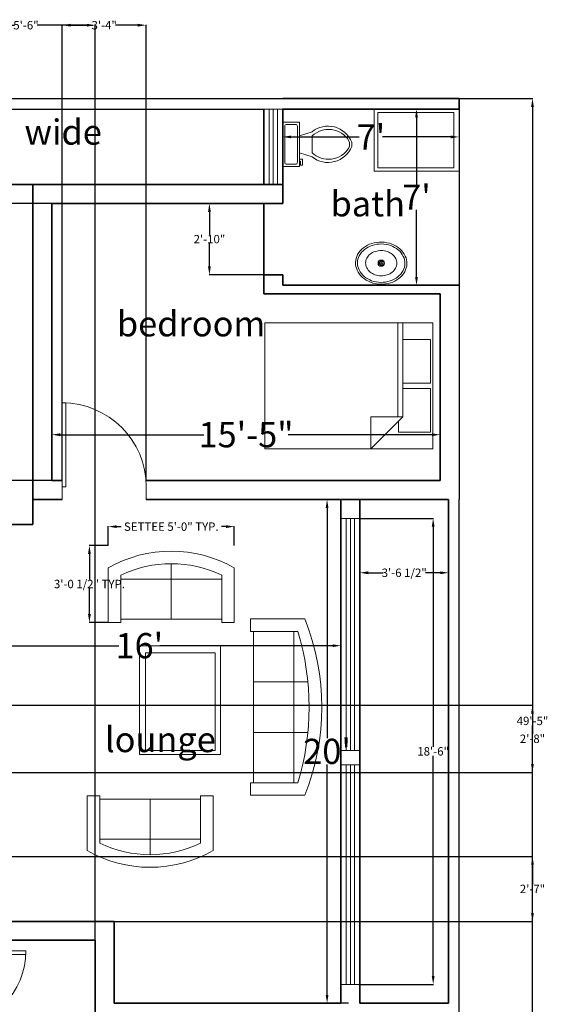
# Model space of a CAD drawing. Units: inches. Extents: x -346 to 220, y 97 to 877.
# Tile 4 of 4: x -32 to 220, y 404 to 873. Entities that reach past the tile are written whole.
import ezdxf

# ---------------------------------------------------------------- set-up
doc = ezdxf.new("R2010")
doc.units = ezdxf.units.IN
doc.header["$MEASUREMENT"] = 0
doc.layers.get('0').update_dxf_attribs({"color": 3})
for name, color, linetype, lineweight in [('A-AREA-IDEN', 130, 'Continuous', 25), ('A-FLOR-FIXT', 9, 'Continuous', 18), ('A-FURN', 8, 'Continuous', 18), ('A-WALL', 7, 'Continuous', 35), ('C-PROP', 94, 'Continuous', 25), ('dim', 170, 'Continuous', 13), ('door', 20, 'Continuous', 18), ('window', 230, 'Continuous', 18)]:
    doc.layers.add(name, color=color, linetype=linetype, lineweight=lineweight)
doc.styles.get("Standard").update_dxf_attribs({"font": 'arial.ttf'})
doc.dimstyles.get("Standard").update_dxf_attribs({"dimtxt": 4, "dimasz": 4, "dimexe": 0.18, "dimexo": 0.0625, "dimgap": 0.09, "dimtad": 0, "dimtih": 1, "dimtoh": 1, "dimdec": 0, "dimzin": 0, "dimdsep": 46, "dimlunit": 3, "dimtxsty": 'Standard', "dimcen": 0.09, "dimadec": 0, "dimazin": 0, "dimtfac": 1, "dimtdec": 0, "dimtofl": 0, "dimtmove": 0, "dimatfit": 3, "dimfxl": 1, "dimtolj": 1, "dimtzin": 0, "dimarcsym": 0})

# ---------------------------------------------------------------- blocks, each defined once
blk = doc.blocks.new('*D2')
at = {"layer": 'Defpoints', "color": 0, "transparency": 16777216}
for p in [(-16.93, 675.59), (-16.93, 653.75), (168.07, 653.75)]:
    blk.add_point(p, dxfattribs=at)
at = {"layer": 'dim', "color": 0, "lineweight": -2, "transparency": 16777216}
for p, q in [((-16.93, 653.81), (-16.93, 675.77)), ((-12.93, 675.59), (55.44, 675.59)), ((164.07, 675.59), (95.71, 675.59)), ((168.07, 653.81), (168.07, 675.77))]:
    blk.add_line(p, q, dxfattribs=at)
at = {"layer": 'dim', "color": 0, "transparency": 16777216}
for points in [[(-12.93, 676.25), (-12.93, 674.92), (-16.93, 675.59)], [(164.07, 676.25), (164.07, 674.92), (168.07, 675.59)]]:
    blk.add_solid(points, dxfattribs=at)
at = {"layer": 'dim', "color": 0, "transparency": 16777216, "insert": (75.57, 675.59), "char_height": 4, "attachment_point": 5}
blk.add_mtext('\\A1;{\\H3x;15\'-5"}', dxfattribs=at)
blk = doc.blocks.new('*D3')
at = {"layer": 'Defpoints', "color": 0, "transparency": 16777216}
for p in [(93.07, 826.04), (177.07, 826.04), (177.07, 817.44)]:
    blk.add_point(p, dxfattribs=at)
at = {"layer": 'dim', "color": 0, "lineweight": -2, "transparency": 16777216}
for p, q in [((93.07, 825.98), (93.07, 817.26)), ((177.07, 825.98), (177.07, 817.26)), ((97.07, 817.44), (129.51, 817.44)), ((173.07, 817.44), (140.63, 817.44))]:
    blk.add_line(p, q, dxfattribs=at)
at = {"layer": 'dim', "color": 0, "transparency": 16777216}
for points in [[(97.07, 818.11), (97.07, 816.78), (93.07, 817.44)], [(173.07, 818.11), (173.07, 816.78), (177.07, 817.44)]]:
    blk.add_solid(points, dxfattribs=at)
at = {"layer": 'dim', "color": 0, "transparency": 16777216, "insert": (135.07, 817.44), "char_height": 4, "attachment_point": 5}
blk.add_mtext("\\A1;{\\H3x;7'}", dxfattribs=at)
blk = doc.blocks.new('*D4')
at = {"layer": 'Defpoints', "color": 0, "transparency": 16777216}
for p in [(177.07, 830.75), (156.76, 746.75), (177.07, 746.75)]:
    blk.add_point(p, dxfattribs=at)
at = {"layer": 'dim', "color": 0, "lineweight": -2, "transparency": 16777216}
for p, q in [((177.01, 830.75), (156.58, 830.75)), ((156.76, 826.75), (156.76, 794.84)), ((156.76, 750.75), (156.76, 782.66)), ((177.01, 746.75), (156.58, 746.75))]:
    blk.add_line(p, q, dxfattribs=at)
at = {"layer": 'dim', "color": 0, "transparency": 16777216}
for points in [[(156.09, 826.75), (157.42, 826.75), (156.76, 830.75)], [(156.09, 750.75), (157.42, 750.75), (156.76, 746.75)]]:
    blk.add_solid(points, dxfattribs=at)
at = {"layer": 'dim', "color": 0, "transparency": 16777216, "insert": (156.76, 788.75), "char_height": 4, "attachment_point": 5}
blk.add_mtext("\\A1;{\\H3x;7'}", dxfattribs=at)
blk = doc.blocks.new('*D5')
at = {"layer": 'Defpoints', "color": 0, "transparency": 16777216}
for p in [(124.4, 644.75), (114.18, 404.75), (124.4, 404.75)]:
    blk.add_point(p, dxfattribs=at)
at = {"layer": 'dim', "color": 0, "lineweight": -2, "transparency": 16777216}
for p, q in [((124.33, 644.75), (114, 644.75)), ((114.18, 640.75), (114.18, 530.96)), ((114.18, 408.75), (114.18, 518.53)), ((124.33, 404.75), (114, 404.75))]:
    blk.add_line(p, q, dxfattribs=at)
at = {"layer": 'dim', "color": 0, "transparency": 16777216}
for points in [[(113.52, 640.75), (114.85, 640.75), (114.18, 644.75)], [(113.52, 408.75), (114.85, 408.75), (114.18, 404.75)]]:
    blk.add_solid(points, dxfattribs=at)
at = {"layer": 'dim', "color": 0, "transparency": 16777216, "insert": (114.18, 524.75), "char_height": 4, "attachment_point": 5}
blk.add_mtext("\\A1;{\\H3x;20'}", dxfattribs=at)
blk = doc.blocks.new('*D6')
at = {"layer": 'Defpoints', "color": 0, "transparency": 16777216}
for p in [(120.77, 575.08), (-71.23, 560.75), (120.77, 560.75)]:
    blk.add_point(p, dxfattribs=at)
at = {"layer": 'dim', "color": 0, "lineweight": -2, "transparency": 16777216}
for p, q in [((-71.23, 560.81), (-71.23, 575.26)), ((-67.23, 575.08), (15.07, 575.08)), ((116.77, 575.08), (34.48, 575.08)), ((120.77, 560.81), (120.77, 575.26))]:
    blk.add_line(p, q, dxfattribs=at)
at = {"layer": 'dim', "color": 0, "transparency": 16777216}
for points in [[(-67.23, 575.75), (-67.23, 574.41), (-71.23, 575.08)], [(116.77, 575.75), (116.77, 574.41), (120.77, 575.08)]]:
    blk.add_solid(points, dxfattribs=at)
at = {"layer": 'dim', "color": 0, "transparency": 16777216, "insert": (24.77, 575.08), "char_height": 4, "attachment_point": 5}
blk.add_mtext("\\A1;{\\H3x;16'}", dxfattribs=at)
blk = doc.blocks.new('*U13')
for p, q in [((0, 0), (0, -6)), ((36, 0), (36, -6))]:
    blk.add_line(p, q)
blk.add_lwpolyline([(0, 0), (0, 36), (1.75, 36), (1.75, 0)], close=True)
blk.add_arc((0, 0), 36, 0, 90)
blk = doc.blocks.new('*U18')
for p, q in [((0, 0), (0, -6)), ((-40, 0), (-40, -6))]:
    blk.add_line(p, q)
blk.add_lwpolyline([(0, 0), (0, 40), (-1.75, 40), (-1.75, 0)], close=True)
blk.add_arc((0, 0), 40, 90, 180)
blk = doc.blocks.new('Bed - Queen')
for p, q in [((0, -80.00003), (0, 0)), ((0, 0), (59.99999, 0)), ((59.99999, 0), (59.99999, -80.00003)), ((7.99999, -1.2), (28.79998, -1.2)), ((7.99999, -14.4), (7.99999, -1.2)), ((28.79998, -1.2), (28.79998, -14.4)), ((31.19999, -1.2), (51.99999, -1.2)), ((31.19999, -14.4), (31.19999, -1.2)), ((51.99999, -1.2), (51.99999, -16.4)), ((0, -14.4), (44.8, -14.4)), ((44.8, -16.8), (0, -16.8)), ((59.99999, -29.6), (44.8, -14.4)), ((44.8, -14.4), (44.8, -29.6)), ((51.99999, -16.4), (46.79936, -16.4)), ((44.8, -29.6), (59.99999, -29.6)), ((59.99999, -80.00003), (0, -80.00003))]:
    blk.add_line(p, q)
blk = doc.blocks.new('Toilet - top')
for p, q in [((9.5, -6), (9.5, -2)), ((-10, -8.5), (-8, -8.5)), ((-10, -9.5), (-10, -8.5)), ((-8, -8.5), (-8, -8)), ((-7, -8), (-7, -9.5)), ((-4, -8), (-6, -14)), ((4, -8), (6, -14)), ((-7, -9.5), (-10, -9.5)), ((4, -14), (-4, -14))]:
    blk.add_line(p, q)
blk.add_lwpolyline([(10.5, -8), (10.5, 0), (-10.5, 0), (-10.5, -8)], close=True)
for points in [[(-9.5, -2), (-9.5, -6)], [(8.5, -1), (-8.5, -1)], [(-8.5, -7), (8.5, -7)]]:
    blk.add_lwpolyline(points)
for centre, radius, start, end in [((-8.62, -1.88), 0.884, 81.8699, 188.1301), ((8.62, -1.88), 0.884, 351.8699, 98.1301), ((-8.62, -6.12), 0.884, 171.8699, 278.1301), ((8.62, -6.12), 0.884, 261.8699, 8.1301), ((3.52, -21.58), 12.17, 141.4691, 247.9714), ((4.2, -21.82), 11.33, 136.3677, 238.9468), ((-3.52, -21.58), 12.17, 292.0284, 38.5307), ((-4.2, -21.82), 11.33, 301.053, 43.6321), ((0, -27.88), 4, 245.7318, 294.2682), ((0, -29), 4, 254.8605, 285.1395)]:
    blk.add_arc(centre, radius, start, end)
blk = doc.blocks.new('Sofa - Roundback 7 ft.')
for p, q in [((-12.00002, -32.4421), (-12.00003, -6.5971)), ((11.99997, -32.4421), (11.99998, -6.5971)), ((-36.000027, -34), (-36.000027, -11.4696)), ((-35.999844, -13.3819), (35.9998, -13.3819)), ((35.99998, -34), (35.99998, -11.4696)), ((-36.000027, -32.4421), (35.99998, -32.4421))]:
    blk.add_line(p, q)
for points in [[(-36.000027, -34), (-42.000027, -34), (-42.000027, -8)], [(41.99998, -8), (41.99998, -34), (35.99998, -34)]]:
    blk.add_lwpolyline(points)
for centre, radius, start, end in [((0, -114.25), 114.25, 68.43141, 111.5686), ((-0.00001, -127.1968), 121.1968, 72.72033, 107.2797)]:
    blk.add_arc(centre, radius, start, end)
blk = doc.blocks.new('Sofa - Roundback Loveseat 5 ft.')
for p, q in [((0, -32.44198), (0, -5.99998)), ((-24, -33.99998), (-24, -11.46958)), ((-23.9998, -13.38178), (23.99986, -13.38178)), ((24.00004, -33.99998), (24.00004, -11.46958)), ((-24, -32.44198), (24.00004, -32.44198))]:
    blk.add_line(p, q)
for points in [[(-24, -33.99998), (-30, -33.99998), (-30, -7.99998)], [(30.00004, -7.99998), (30.00004, -33.99998), (24.00004, -33.99998)]]:
    blk.add_lwpolyline(points)
for centre, radius, start, end in [((0, -60.24998), 60.24998, 60.13715, 119.8628), ((0, -61.38438), 55.38444, 64.32083, 115.6792)]:
    blk.add_arc(centre, radius, start, end)
blk = doc.blocks.new('Sink - Oval top')
for p, q in [((-1, 0), (1, 0)), ((0, 1), (0, -1))]:
    blk.add_line(p, q)
for points in [[(-12.23, 0.39, 0.117634), (-11.46, -3.36, 0.104469), (-8.88, -6.8, 0.090016), (-5.08, -9.07, 0.08192), (-0.32, -10.02, 0.08192), (4.49, -9.38, 0.090016), (8.42, -7.36, 0.104469), (11.22, -4.09, 0.117634), (12.23, -0.39, 0.117634), (11.46, 3.36, 0.104469), (8.88, 6.8, 0.090016), (5.08, 9.07, 0.08192), (0.32, 10.02, 0.08192), (-4.49, 9.38, 0.090016), (-8.42, 7.36, 0.104469), (-11.22, 4.09, 0.117634)], [(-11.29, 0.16, 0.118622), (-10.52, -3.25, 0.104678), (-8.07, -6.36, 0.089562), (-4.54, -8.37, 0.081185), (-0.13, -9.15, 0.081185), (4.3, -8.49, 0.089562), (7.89, -6.58, 0.104678), (10.42, -3.55, 0.118622), (11.29, -0.16, 0.118622), (10.52, 3.25, 0.104678), (8.07, 6.36, 0.089562), (4.54, 8.37, 0.081185), (0.13, 9.15, 0.081185), (-4.3, 8.49, 0.089562), (-7.89, 6.58, 0.104678), (-10.42, 3.55, 0.118622)], [(-7.42, 0.08, 0.118283), (-6.91, -2.17, 0.104607), (-5.29, -4.21, 0.089718), (-2.97, -5.53, 0.081436), (-0.07, -6.04, 0.081436), (2.84, -5.59, 0.089718), (5.2, -4.33, 0.104607), (6.86, -2.32, 0.118283), (7.42, -0.08, 0.118283), (6.91, 2.17, 0.104607), (5.29, 4.21, 0.089718), (2.97, 5.53, 0.081436), (0.07, 6.04, 0.081436), (-2.84, 5.59, 0.089718), (-5.2, 4.33, 0.104607), (-6.86, 2.32, 0.118283)]]:
    blk.add_lwpolyline(points, format="xyb", close=True)
for radius in [1.5, 1]:
    blk.add_circle((0, 0), radius)
blk = doc.blocks.new('WIN-36x9-PLAN')
for p, q in [((2.5, 36), (2.5, 0)), ((4.5, 36), (4.5, 0)), ((6.5, 36), (6.5, 0))]:
    blk.add_line(p, q)
blk.add_lwpolyline([(0, 36), (9, 36), (9, 0), (0, 0)], close=True)
blk = doc.blocks.new('TABLE-COFFEE-RECT')
for points in [[(0, 51.83), (38.64, 51.83), (38.64, 0), (0, 0)], [(2.97, 48.5), (36.03, 48.5), (36.03, 1.93), (2.97, 1.93)]]:
    blk.add_lwpolyline(points, close=True)
blk = doc.blocks.new('*D38')
at = {"layer": 'Defpoints', "color": 0, "transparency": 16777216}
for p in [(69.99, 631.8), (9.99, 622.8), (69.99, 622.8)]:
    blk.add_point(p, dxfattribs=at)
at = {"layer": 'dim', "color": 0, "lineweight": -2, "transparency": 16777216}
for p, q in [((9.99, 622.87), (9.99, 631.98)), ((13.99, 631.8), (16.07, 631.8)), ((65.99, 631.8), (63.9, 631.8)), ((69.99, 622.87), (69.99, 631.98))]:
    blk.add_line(p, q, dxfattribs=at)
at = {"layer": 'dim', "color": 0, "transparency": 16777216}
for points in [[(13.99, 632.47), (13.99, 631.14), (9.99, 631.8)], [(65.99, 632.47), (65.99, 631.14), (69.99, 631.8)]]:
    blk.add_solid(points, dxfattribs=at)
at = {"layer": 'dim', "color": 0, "transparency": 16777216, "insert": (39.99, 631.8), "char_height": 4, "attachment_point": 5}
blk.add_mtext('\\A1;SETTEE 5\'-0" TYP.', dxfattribs=at)
blk = doc.blocks.new('*D39')
at = {"layer": 'Defpoints', "color": 0, "transparency": 16777216}
for p in [(0.99, 622.8), (9.99, 622.8), (9.99, 586.14)]:
    blk.add_point(p, dxfattribs=at)
at = {"layer": 'dim', "color": 0, "lineweight": -2, "transparency": 16777216}
for p, q in [((9.92, 622.8), (0.81, 622.8)), ((0.99, 618.8), (0.99, 606.63)), ((0.99, 590.14), (0.99, 602.31)), ((9.92, 586.14), (0.81, 586.14))]:
    blk.add_line(p, q, dxfattribs=at)
at = {"layer": 'dim', "color": 0, "transparency": 16777216}
for points in [[(0.32, 618.8), (1.65, 618.8), (0.99, 622.8)], [(0.32, 590.14), (1.65, 590.14), (0.99, 586.14)]]:
    blk.add_solid(points, dxfattribs=at)
at = {"layer": 'dim', "color": 0, "transparency": 16777216, "insert": (0.99, 604.47), "char_height": 4, "attachment_point": 5}
blk.add_mtext('\\A1;3\'-0 1/2" TYP.', dxfattribs=at)
blk = doc.blocks.new('*D51')
at = {"layer": 'Defpoints', "color": 0, "transparency": 16777216}
for p in [(177.07, 835.75), (212, 835.75), (177.07, 242.75)]:
    blk.add_point(p, dxfattribs=at)
at = {"layer": 'dim', "color": 0, "lineweight": -2, "transparency": 16777216}
for p, q in [((177.13, 835.75), (212.18, 835.75)), ((212, 831.75), (212, 541.38)), ((212, 246.75), (212, 537.11)), ((177.13, 242.75), (212.18, 242.75))]:
    blk.add_line(p, q, dxfattribs=at)
at = {"layer": 'dim', "color": 0, "transparency": 16777216}
for points in [[(211.33, 831.75), (212.66, 831.75), (212, 835.75)], [(211.33, 246.75), (212.66, 246.75), (212, 242.75)]]:
    blk.add_solid(points, dxfattribs=at)
at = {"layer": 'dim', "color": 0, "transparency": 16777216, "insert": (212, 539.25), "char_height": 4, "attachment_point": 5}
blk.add_mtext('\\A1;49\'-5"', dxfattribs=at)
blk = doc.blocks.new('*D56')
at = {"layer": 'Defpoints', "color": 0, "transparency": 16777216}
for p in [(-51.85, 785.75), (-16.93, 785.75), (-16.93, 653.75)]:
    blk.add_point(p, dxfattribs=at)
at = {"layer": 'dim', "color": 0, "lineweight": -2, "transparency": 16777216}
for p, q in [((-16.99, 785.75), (-52.03, 785.75)), ((-51.85, 781.75), (-51.85, 721.88)), ((-51.85, 657.75), (-51.85, 717.61)), ((-16.99, 653.75), (-52.03, 653.75))]:
    blk.add_line(p, q, dxfattribs=at)
at = {"layer": 'dim', "color": 0, "transparency": 16777216}
for points in [[(-52.52, 781.75), (-51.19, 781.75), (-51.85, 785.75)], [(-52.52, 657.75), (-51.19, 657.75), (-51.85, 653.75)]]:
    blk.add_solid(points, dxfattribs=at)
at = {"layer": 'dim', "color": 0, "transparency": 16777216, "insert": (-51.85, 719.75), "char_height": 4, "attachment_point": 5}
blk.add_mtext('\\A1;11\'-0"', dxfattribs=at)
blk = doc.blocks.new('*D58')
at = {"layer": 'Defpoints', "color": 0, "transparency": 16777216}
for p in [(3.77, 870.67), (3.77, 341.75), (-62.23, 331.75)]:
    blk.add_point(p, dxfattribs=at)
at = {"layer": 'dim', "color": 0, "lineweight": -2, "transparency": 16777216}
for p, q in [((-62.23, 331.81), (-62.23, 870.85)), ((-58.23, 870.67), (-34.63, 870.67)), ((-0.23, 870.67), (-23.82, 870.67)), ((3.77, 341.81), (3.77, 870.85))]:
    blk.add_line(p, q, dxfattribs=at)
at = {"layer": 'dim', "color": 0, "transparency": 16777216}
for points in [[(-58.23, 871.34), (-58.23, 870), (-62.23, 870.67)], [(-0.23, 871.34), (-0.23, 870), (3.77, 870.67)]]:
    blk.add_solid(points, dxfattribs=at)
at = {"layer": 'dim', "color": 0, "transparency": 16777216, "insert": (-29.23, 870.67), "char_height": 4, "attachment_point": 5}
blk.add_mtext('\\A1;5\'-6"', dxfattribs=at)
blk = doc.blocks.new('*D60')
at = {"layer": 'Defpoints', "color": 0, "transparency": 16777216}
for p in [(129.77, 644.75), (172.07, 644.75), (129.77, 609.82)]:
    blk.add_point(p, dxfattribs=at)
at = {"layer": 'dim', "color": 0, "lineweight": -2, "transparency": 16777216}
for p, q in [((129.77, 644.68), (129.77, 609.64)), ((172.07, 644.68), (172.07, 609.64)), ((133.77, 609.82), (140.86, 609.82)), ((168.07, 609.82), (160.99, 609.82))]:
    blk.add_line(p, q, dxfattribs=at)
at = {"layer": 'dim', "color": 0, "transparency": 16777216}
for points in [[(133.77, 610.49), (133.77, 609.15), (129.77, 609.82)], [(168.07, 610.49), (168.07, 609.15), (172.07, 609.82)]]:
    blk.add_solid(points, dxfattribs=at)
at = {"layer": 'dim', "color": 0, "transparency": 16777216, "insert": (150.92, 609.82), "char_height": 4, "attachment_point": 5}
blk.add_mtext('\\A1;3\'-6 1/2"', dxfattribs=at)
blk = doc.blocks.new('*D63')
at = {"layer": 'Defpoints', "color": 0, "transparency": 16777216}
for p in [(-71.23, 546.75), (212, 546.75), (-71.23, 514.75)]:
    blk.add_point(p, dxfattribs=at)
at = {"layer": 'dim', "color": 0, "lineweight": -2, "transparency": 16777216}
for p, q in [((-71.16, 546.75), (212.18, 546.75)), ((212, 542.75), (212, 532.88)), ((212, 518.75), (212, 528.61)), ((-71.16, 514.75), (212.18, 514.75))]:
    blk.add_line(p, q, dxfattribs=at)
at = {"layer": 'dim', "color": 0, "transparency": 16777216}
for points in [[(211.33, 542.75), (212.66, 542.75), (212, 546.75)], [(211.33, 518.75), (212.66, 518.75), (212, 514.75)]]:
    blk.add_solid(points, dxfattribs=at)
at = {"layer": 'dim', "color": 0, "transparency": 16777216, "insert": (212, 530.75), "char_height": 4, "attachment_point": 5}
blk.add_mtext('\\A1;2\'-8"', dxfattribs=at)
blk = doc.blocks.new('*D65')
at = {"layer": 'Defpoints', "color": 0, "transparency": 16777216}
for p in [(27.96, 870.67), (-11.93, 653.75), (27.96, 653.75)]:
    blk.add_point(p, dxfattribs=at)
at = {"layer": 'dim', "color": 0, "lineweight": -2, "transparency": 16777216}
for p, q in [((-11.93, 653.81), (-11.93, 870.85)), ((-7.93, 870.67), (2.61, 870.67)), ((23.96, 870.67), (13.42, 870.67)), ((27.96, 653.81), (27.96, 870.85))]:
    blk.add_line(p, q, dxfattribs=at)
at = {"layer": 'dim', "color": 0, "transparency": 16777216}
for points in [[(-7.93, 871.34), (-7.93, 870), (-11.93, 870.67)], [(23.96, 871.34), (23.96, 870), (27.96, 870.67)]]:
    blk.add_solid(points, dxfattribs=at)
at = {"layer": 'dim', "color": 0, "transparency": 16777216, "insert": (8.02, 870.67), "char_height": 4, "attachment_point": 5}
blk.add_mtext('\\A1;3\'-4"', dxfattribs=at)
blk = doc.blocks.new('*D67')
at = {"layer": 'Defpoints', "color": 0, "transparency": 16777216}
for p in [(58.15, 785.75), (93.07, 785.75), (93.07, 751.75)]:
    blk.add_point(p, dxfattribs=at)
at = {"layer": 'dim', "color": 0, "lineweight": -2, "transparency": 16777216}
for p, q in [((93.01, 785.75), (57.97, 785.75)), ((58.15, 781.75), (58.15, 770.88)), ((58.15, 755.75), (58.15, 766.61)), ((93.01, 751.75), (57.97, 751.75))]:
    blk.add_line(p, q, dxfattribs=at)
at = {"layer": 'dim', "color": 0, "transparency": 16777216}
for points in [[(57.48, 781.75), (58.81, 781.75), (58.15, 785.75)], [(57.48, 755.75), (58.81, 755.75), (58.15, 751.75)]]:
    blk.add_solid(points, dxfattribs=at)
at = {"layer": 'dim', "color": 0, "transparency": 16777216, "insert": (58.15, 768.75), "char_height": 4, "attachment_point": 5}
blk.add_mtext('\\A1;2\'-10"', dxfattribs=at)
blk = doc.blocks.new('*D70')
at = {"layer": 'Defpoints', "color": 0, "transparency": 16777216}
for p in [(129.77, 635.75), (129.77, 413.75), (164.7, 413.75)]:
    blk.add_point(p, dxfattribs=at)
at = {"layer": 'dim', "color": 0, "lineweight": -2, "transparency": 16777216}
for p, q in [((129.84, 635.75), (164.88, 635.75)), ((164.7, 631.75), (164.7, 526.88)), ((164.7, 417.75), (164.7, 522.61)), ((129.84, 413.75), (164.88, 413.75))]:
    blk.add_line(p, q, dxfattribs=at)
at = {"layer": 'dim', "color": 0, "transparency": 16777216}
for points in [[(164.03, 631.75), (165.37, 631.75), (164.7, 635.75)], [(164.03, 417.75), (165.37, 417.75), (164.7, 413.75)]]:
    blk.add_solid(points, dxfattribs=at)
at = {"layer": 'dim', "color": 0, "transparency": 16777216, "insert": (164.7, 524.75), "char_height": 4, "attachment_point": 5}
blk.add_mtext('\\A1;18\'-6"', dxfattribs=at)
blk = doc.blocks.new('*D72')
at = {"layer": 'Defpoints', "color": 0, "transparency": 16777216}
for p in [(-118.63, 474.69), (212, 474.69), (-80.23, 443.75)]:
    blk.add_point(p, dxfattribs=at)
at = {"layer": 'dim', "color": 0, "lineweight": -2, "transparency": 16777216}
for p, q in [((-118.57, 474.69), (212.18, 474.69)), ((212, 470.69), (212, 461.32)), ((212, 447.75), (212, 457.12)), ((-80.16, 443.75), (212.18, 443.75))]:
    blk.add_line(p, q, dxfattribs=at)
at = {"layer": 'dim', "color": 0, "transparency": 16777216}
for points in [[(211.33, 470.69), (212.66, 470.69), (212, 474.69)], [(211.33, 447.75), (212.66, 447.75), (212, 443.75)]]:
    blk.add_solid(points, dxfattribs=at)
at = {"layer": 'dim', "color": 0, "transparency": 16777216, "insert": (212, 459.22), "char_height": 4, "attachment_point": 5}
blk.add_mtext('\\A1;2\'-7"', dxfattribs=at)

msp = doc.modelspace()

# ---------------------------------------------------------------- linework, layer by layer
at = {"layer": 'A-FLOR-FIXT'}
for points in [[(177.07, 830.75), (136.58, 830.75), (136.58, 801.1), (177.07, 801.1)], [(174.6, 829.05), (138.3, 829.05), (138.3, 802.68), (174.6, 802.68)]]:
    msp.add_lwpolyline(points, close=True, dxfattribs=at)
at = {"layer": 'A-WALL'}
for p, q in [((177.07, 835.75), (93.07, 835.75)), ((177.07, 830.75), (177.07, 835.75)), ((84.07, 830.75), (84.07, 794.75)), ((93.07, 830.75), (93.07, 794.75)), ((93.07, 830.75), (177.07, 830.75)), ((-227.93, 794.75), (93.07, 794.75)), ((-25.93, 794.75), (-25.93, 632.75)), ((93.07, 794.75), (93.07, 785.75)), ((-16.93, 653.75), (-16.93, 785.75)), ((-16.93, 785.75), (84.07, 785.75)), ((84.07, 785.75), (84.07, 742.75)), ((93.07, 785.75), (84.07, 785.75)), ((93.07, 751.75), (84.07, 751.75)), ((93.07, 746.75), (93.07, 751.75)), ((93.07, 746.75), (177.07, 746.75)), ((84.07, 742.75), (168.07, 742.75)), ((168.07, 742.75), (168.07, 653.75)), ((-11.93, 653.75), (-16.93, 653.75)), ((168.07, 653.75), (27.96, 653.75)), ((-11.93, 644.75), (-25.93, 644.75)), ((172.07, 644.75), (28.07, 644.75)), ((120.77, 404.75), (120.77, 644.75)), ((129.77, 404.75), (129.77, 644.75)), ((172.07, 404.75), (172.07, 644.75)), ((-25.93, 632.75), (-39.93, 632.75)), ((-71.23, 443.75), (12.77, 443.75)), ((12.77, 443.75), (12.77, 404.75)), ((-62.23, 434.75), (3.77, 434.75)), ((3.77, 434.75), (3.77, 390.75)), ((3.77, 434.75), (3.77, 390.75)), ((120.77, 404.75), (12.77, 404.75)), ((172.07, 404.75), (129.77, 404.75))]:
    msp.add_line(p, q, dxfattribs=at)
at = {"layer": 'C-PROP'}
for p, q in [((-298.95, 835.75), (177.07, 835.75)), ((177.07, 835.75), (177.07, 644.75)), ((-293.95, 830.75), (84.07, 830.75)), ((177.07, 138.35), (177.07, 644.75))]:
    msp.add_line(p, q, dxfattribs=at)
at = {"layer": 'door'}
msp.add_line((-11.93, 653.75), (-11.93, 644.75), dxfattribs=at)
at = {"layer": 'window'}
for p, q in [((129.77, 635.75), (120.77, 635.75)), ((123.27, 635.75), (123.27, 525.12)), ((125.27, 635.75), (125.27, 525.12)), ((127.27, 635.75), (127.27, 525.12)), ((123.27, 518.37), (123.27, 413.75)), ((125.27, 518.37), (125.27, 413.75)), ((127.27, 518.37), (127.27, 413.75)), ((129.77, 413.75), (120.77, 413.75))]:
    msp.add_line(p, q, dxfattribs=at)
msp.add_lwpolyline([(120.77, 521.75), (120.77, 525.12), (129.77, 525.12), (129.77, 521.75), (129.77, 518.37), (120.77, 518.37)], close=True, dxfattribs=at)

# ---------------------------------------------------------------- block references
at = {"layer": 'A-FLOR-FIXT', "rotation": 90}
msp.add_blockref('Toilet - top', (93.03, 813.93), dxfattribs=at)
at = {"layer": 'A-FLOR-FIXT'}
msp.add_blockref('Sink - Oval top', (139.95, 757.31), dxfattribs=at)
at = {"layer": 'A-FURN'}
for name, p, rotation in [('Bed - Queen', (164.6, 728.87), 270), ('Sofa - Roundback 7 ft.', (111.65, 545.8), 270), ('Sofa - Roundback Loveseat 5 ft.', (29.89, 469.51), 180)]:
    msp.add_blockref(name, p, dxfattribs=dict(at, rotation=rotation))
for name, p in [('Sofa - Roundback Loveseat 5 ft.', (39.99, 620.14)), ('TABLE-COFFEE-RECT', (24.77, 523.25))]:
    msp.add_blockref(name, p, dxfattribs=at)
at = {"layer": 'door', "xscale": -1}
msp.add_blockref('*U18', (-11.93, 650.75), dxfattribs=at)
at = {"layer": 'door', "rotation": 270}
msp.add_blockref('*U13', (-65.23, 429.75), dxfattribs=at)
at = {"layer": 'window'}
msp.add_blockref('WIN-36x9-PLAN', (84.07, 794.75), dxfattribs=at)

# ---------------------------------------------------------------- texts
at = {"layer": 'A-AREA-IDEN', "char_height": 12, "attachment_point": 1}
for s, insert in [('wide', (-29.95, 825.75)), ('bath', (115.83, 791.59)), ('bedroom', (14.07, 734.43)), ('lounge', (8.37, 536.38))]:
    msp.add_mtext_dynamic_manual_height_columns(s, width=62.6765, gutter_width=1, heights=[0], dxfattribs=dict(at, insert=insert))

# ---------------------------------------------------------------- dimensions: what is measured, and where the dimension line sits
at = {"layer": 'dim'}
for base, p1, p2, picture, middle in [((3.77, 870.67), (-62.23, 331.75), (3.77, 341.75), '*D58', (-29.23, 870.67)), ((27.96, 870.67), (-11.93, 653.75), (27.96, 653.75), '*D65', (8.02, 870.67))]:
    dim = msp.add_linear_dim(base=base, p1=p1, p2=p2, dimstyle='Standard', override={"dimdec": 1, "dimlfac": 1, "dimrnd": 0, "dimzin": 1, "dimdsep": 46, "dimlunit": 4, "dimfrac": 2}, dxfattribs=at)
    dim.commit()
    dim.dimension.update_dxf_attribs({"geometry": picture, "text_midpoint": middle})
for base, p1, p2, angle, picture, middle in [((212, 835.75), (177.07, 242.75), (177.07, 835.75), 90, '*D51', (212, 539.25)), ((-51.85, 785.75), (-16.93, 653.75), (-16.93, 785.75), 90, '*D56', (-51.85, 719.75)), ((58.15, 785.75), (93.07, 751.75), (93.07, 785.75), 90, '*D67', (58.15, 768.75)), ((129.77, 609.82), (172.07, 644.75), (129.77, 644.75), 180, '*D60', (150.92, 609.82)), ((164.7, 413.75), (129.77, 635.75), (129.77, 413.75), 270, '*D70', (164.7, 524.75)), ((212, 546.75), (-71.23, 514.75), (-71.23, 546.75), 90, '*D63', (212, 530.75)), ((212, 474.69), (-80.23, 443.75), (-118.63, 474.69), 90, '*D72', (212, 459.22))]:
    dim = msp.add_linear_dim(base=base, p1=p1, p2=p2, angle=angle, dimstyle='Standard', override={"dimdec": 1, "dimlfac": 1, "dimrnd": 0, "dimzin": 1, "dimdsep": 46, "dimlunit": 4, "dimfrac": 2}, dxfattribs=at)
    dim.commit()
    dim.dimension.update_dxf_attribs({"geometry": picture, "text_midpoint": middle})
for base, p1, p2, text, override, picture, middle in [((156.76, 746.75), (177.07, 830.75), (177.07, 746.75), '{\\H3x;<>}', {"dimclrd": 0, "dimclre": 0, "dimclrt": 0}, '*D4', (156.76, 788.75)), ((114.18, 404.75), (124.4, 644.75), (124.4, 404.75), '{\\H3x;<>}', {"dimclrd": 0, "dimclre": 0, "dimclrt": 0}, '*D5', (114.18, 524.75)), ((0.99, 622.8), (9.99, 586.14), (9.99, 622.8), '<> TYP.', {"dimdec": 1, "dimlfac": 1, "dimrnd": 0, "dimzin": 1, "dimdsep": 46, "dimlunit": 4, "dimfrac": 2}, '*D39', (0.99, 604.47))]:
    dim = msp.add_linear_dim(base=base, p1=p1, p2=p2, angle=90, text=text, dimstyle='Standard', override=override, dxfattribs=at)
    dim.commit()
    dim.dimension.update_dxf_attribs({"geometry": picture, "text_midpoint": middle})
for base, p1, p2, text, override, picture, middle in [((177.07, 817.44), (93.07, 826.04), (177.07, 826.04), '{\\H3x;<>}', {"dimclrd": 0, "dimclre": 0, "dimclrt": 0}, '*D3', (135.07, 817.44)), ((-16.93, 675.59), (168.07, 653.75), (-16.93, 653.75), '{\\H3x;<>}', {"dimclrd": 0, "dimclre": 0, "dimclrt": 0}, '*D2', (75.57, 675.59)), ((69.99, 631.8), (9.99, 622.8), (69.99, 622.8), 'SETTEE <> TYP.', {"dimdec": 1, "dimlfac": 1, "dimrnd": 0, "dimzin": 1, "dimdsep": 46, "dimlunit": 4, "dimfrac": 2}, '*D38', (39.99, 631.8)), ((120.77, 575.08), (-71.23, 560.75), (120.77, 560.75), '{\\H3x;<>}', {"dimclrd": 0, "dimclre": 0, "dimclrt": 0}, '*D6', (24.77, 575.08))]:
    dim = msp.add_linear_dim(base=base, p1=p1, p2=p2, text=text, dimstyle='Standard', override=override, dxfattribs=at)
    dim.commit()
    dim.dimension.update_dxf_attribs({"geometry": picture, "text_midpoint": middle})

doc.saveas('drawing.dxf')
